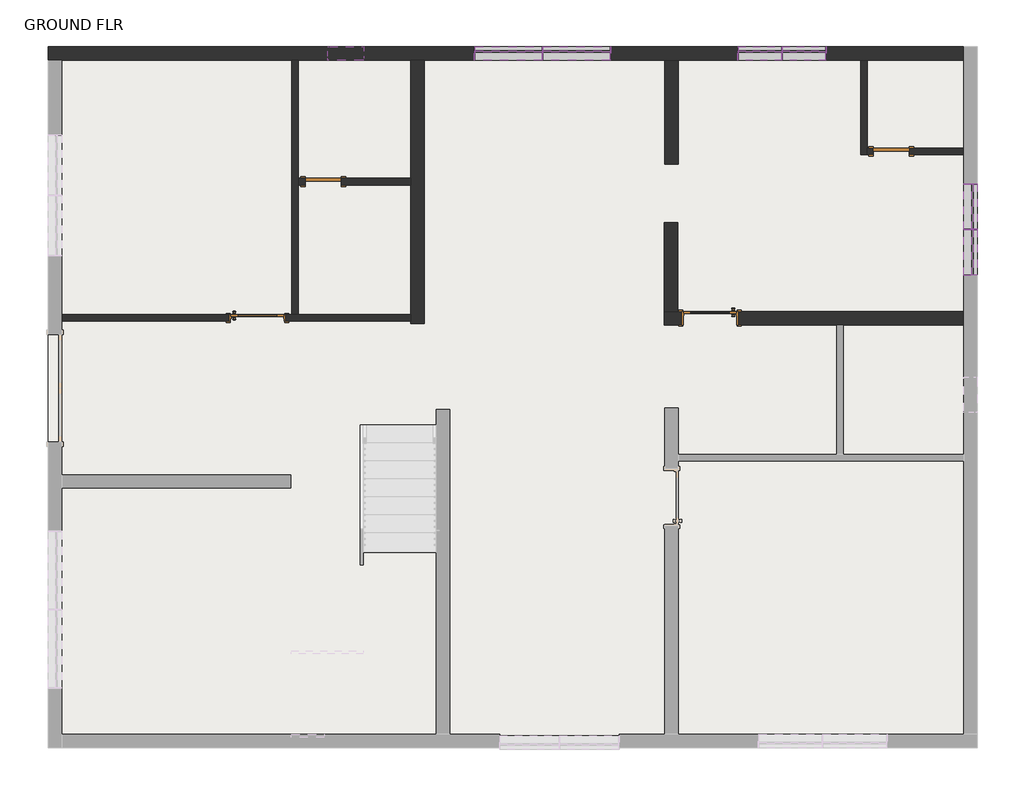
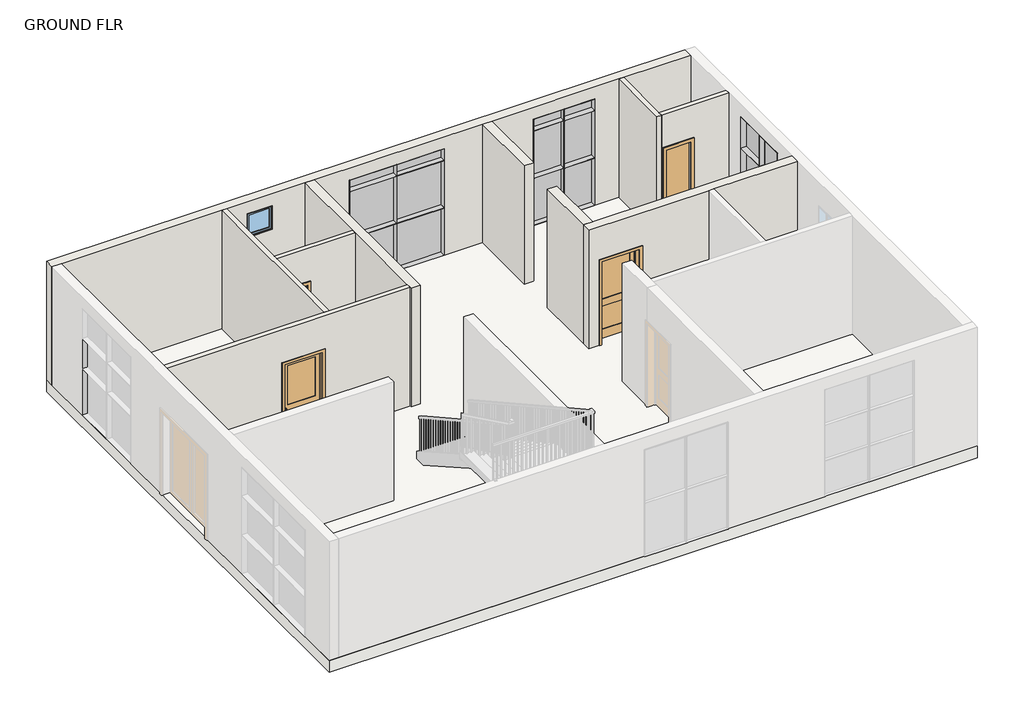
# One storey, part 2 of 3: 53 members, 18 plates, 10 walls, 4 doors, 1 slab, 1 window.
"""IFC4 building model written with IfcOpenShell, lengths in millimetres."""

from ifc_helpers import new_model, si_unit, frame, origin, origin_with_axes, place, context, project, spatial, polyline, outline, extrude, faceted_brep, transform, mapped, element, save
from components import door_interior_single_2_panel_wood_d4071c8b, door_interior_single_2_panel_wood_5dd36918, single_flush_bathroom_2_x_7_0bf9f8da, member_9b8c6d2b, member_330b65be, member_e8dc6119, member_d66a3bdd, member_a87dc375, member_05d02c6e, member_049ff311, member_f4ca0770, member_7d5ce663, member_d90fa784, member_091456ab, member_579a4f36, member_81a97153, member_446da441, member_c9ff8968, member_427a6bf5, member_b53b5e8d, member_fa9cb678, system_panel_glazed_6813505b, system_panel_glazed_75f85cfe, system_panel_glazed_a35be92d, system_panel_glazed_47c35fab, system_panel_glazed_b4a359f9, system_panel_glazed_e62deb46, system_panel_glazed_14aec0f7, system_panel_glazed_b869959d, system_panel_glazed_d22e8d08, window_80340324

model = new_model("IFC4")

# Units and contexts
model_context = context("Model", 3, world=origin())
ifc_project = project(units=[si_unit("LENGTHUNIT", "METRE", prefix="MILLI")], contexts=[model_context])

# Site, building, storey
site = spatial("IfcSite", under=ifc_project)
building = spatial("IfcBuilding", under=site)
storey = spatial("IfcBuildingStorey", under=building, Name="GROUND FLR", Elevation=304.8)

# Doors
placement = place(None, origin())
door_interior_single_2_panel_wood_shape = door_interior_single_2_panel_wood_d4071c8b(model_context)
element("IfcDoor", 1, ObjectType="Door-Interior-Single-2_Panel-Wood", at=placement, inside=storey, context=model_context, shape_type="MappedRepresentation", body=[
    mapped(door_interior_single_2_panel_wood_shape, transform((-6802.5434923, 1073.5921668, 304.8), x_axis=(1.0, 0.0, 0.0), y_axis=(0.0, 1.0, 0.0), z_axis=(0.0, 0.0, 1.0))),
])
door_interior_single_2_panel_wood_2_shape = door_interior_single_2_panel_wood_5dd36918(model_context)
element("IfcDoor", 2, ObjectType="Door-Interior-Single-2_Panel-Wood", at=placement, inside=storey, context=model_context, shape_type="MappedRepresentation", body=[
    mapped(door_interior_single_2_panel_wood_2_shape, transform((872.4132515, 1069.6301442, 304.8), x_axis=(-1.0, 0.0, 0.0), y_axis=(0.0, -1.0, 0.0), z_axis=(0.0, 0.0, 1.0))),
])
single_flush_bathroom_2_x_7_shape = single_flush_bathroom_2_x_7_0bf9f8da(model_context)
element("IfcDoor", 3, ObjectType="Single-Flush : BATHROOM 2' X 7'", at=placement, inside=storey, context=model_context, shape_type="MappedRepresentation", body=[
    mapped(single_flush_bathroom_2_x_7_shape, transform((-5684.9434923, 3381.9805563, 304.8), x_axis=(-1.0, 0.0, 0.0), y_axis=(0.0, -1.0, 0.0), z_axis=(0.0, 0.0, 1.0))),
])
element("IfcDoor", 4, ObjectType="Single-Flush : BATHROOM 2' X 7'", at=placement, inside=storey, context=model_context, shape_type="MappedRepresentation", body=[
    mapped(single_flush_bathroom_2_x_7_shape, transform((3941.8301763, 3897.1946858, 304.8), x_axis=(-1.0, 0.0, 0.0), y_axis=(0.0, -1.0, 0.0), z_axis=(0.0, 0.0, 1.0))),
])

# Members
member_shape = member_9b8c6d2b(model_context)
element("IfcMember", 5, ObjectType="Rectangular Mullion : 2.5\" x 5\" rectangular", at=placement, inside=storey, context=model_context, shape_type="MappedRepresentation", body=[
    mapped(member_shape, transform((-10239.065751, 4179.68206, 1498.6), x_axis=(0.0, 1.0, 0.0), y_axis=(-1.0, 0.0, 0.0), z_axis=(0.0, 0.0, 1.0))),
])
member_2_shape = member_330b65be(model_context)
element("IfcMember", 6, ObjectType="Rectangular Mullion : 2.5\" x 5\" rectangular", at=placement, inside=storey, context=model_context, shape_type="MappedRepresentation", body=[
    mapped(member_2_shape, transform((-10239.065751, 4179.68206, 2273.3), x_axis=(0.0, 1.0, 0.0), y_axis=(-1.0, 0.0, 0.0), z_axis=(0.0, 0.0, 1.0))),
])
member_3_shape = member_e8dc6119(model_context)
element("IfcMember", 7, ObjectType="Rectangular Mullion : 2.5\" x 5\" rectangular", at=placement, inside=storey, context=model_context, shape_type="MappedRepresentation", body=[
    mapped(member_3_shape, transform((5293.034249, 2571.0346634, 2235.2), x_axis=(0.0, -1.0, 0.0), y_axis=(-1.0, 0.0, 0.0), z_axis=(0.0, 0.0, -1.0))),
])
member_4_shape = member_d66a3bdd(model_context)
element("IfcMember", 8, ObjectType="Rectangular Mullion : 2.5\" x 5\" rectangular", at=placement, inside=storey, context=model_context, shape_type="MappedRepresentation", body=[
    mapped(member_4_shape, transform((5293.034249, 3348.9096634, 3048.0), x_axis=(0.0, 1.0, 0.0), y_axis=(-1.0, 0.0, 0.0), z_axis=(0.0, 0.0, 1.0))),
])
element("IfcMember", 9, ObjectType="Rectangular Mullion : 2.5\" x 5\" rectangular", at=placement, inside=storey, context=model_context, shape_type="MappedRepresentation", body=[
    mapped(member_4_shape, transform((5293.034249, 1793.1596634, 2235.2), x_axis=(0.0, -1.0, 0.0), y_axis=(-1.0, 0.0, 0.0), z_axis=(0.0, 0.0, -1.0))),
])
member_5_shape = member_a87dc375(model_context)
element("IfcMember", 10, ObjectType="Rectangular Mullion : 2.5\" x 5\" rectangular", at=placement, inside=storey, context=model_context, shape_type="MappedRepresentation", body=[
    mapped(member_5_shape, transform((5293.034249, 2571.0346634, 304.8), x_axis=(0.0, -1.0, 0.0), y_axis=(-1.0, 0.0, 0.0), z_axis=(0.0, 0.0, -1.0))),
])
member_6_shape = member_05d02c6e(model_context)
element("IfcMember", 11, ObjectType="Rectangular Mullion : 2.5\" x 5\" rectangular", at=placement, inside=storey, context=model_context, shape_type="MappedRepresentation", body=[
    mapped(member_6_shape, transform((5293.034249, 2571.0346634, 1168.4), x_axis=(0.0, -1.0, 0.0), y_axis=(-1.0, 0.0, 0.0), z_axis=(0.0, 0.0, -1.0))),
])
member_7_shape = member_049ff311(model_context)
element("IfcMember", 12, ObjectType="Rectangular Mullion : 2.5\" x 5\" rectangular", at=placement, inside=storey, context=model_context, shape_type="MappedRepresentation", body=[
    mapped(member_7_shape, transform((5293.034249, 1793.1596634, 304.8), x_axis=(0.0, -1.0, 0.0), y_axis=(-1.0, 0.0, 0.0), z_axis=(0.0, 0.0, -1.0))),
])
member_8_shape = member_f4ca0770(model_context)
element("IfcMember", 13, ObjectType="Rectangular Mullion : 2.5\" x 5\" rectangular", at=placement, inside=storey, context=model_context, shape_type="MappedRepresentation", body=[
    mapped(member_8_shape, transform((5293.034249, 3348.9096634, 2235.2), x_axis=(0.0, 1.0, 0.0), y_axis=(-1.0, 0.0, 0.0), z_axis=(0.0, 0.0, 1.0))),
])
element("IfcMember", 14, ObjectType="Rectangular Mullion : 2.5\" x 5\" rectangular", at=placement, inside=storey, context=model_context, shape_type="MappedRepresentation", body=[
    mapped(member_8_shape, transform((5293.034249, 1793.1596634, 1168.4), x_axis=(0.0, -1.0, 0.0), y_axis=(-1.0, 0.0, 0.0), z_axis=(0.0, 0.0, -1.0))),
])
element("IfcMember", 15, ObjectType="Rectangular Mullion : 2.5\" x 5\" rectangular", at=placement, inside=storey, context=model_context, shape_type="MappedRepresentation", body=[
    mapped(member_7_shape, transform((5293.034249, 3348.9096634, 1168.4), x_axis=(0.0, 1.0, 0.0), y_axis=(-1.0, 0.0, 0.0), z_axis=(0.0, 0.0, 1.0))),
])
member_9_shape = member_7d5ce663(model_context)
element("IfcMember", 16, ObjectType="Rectangular Mullion : 2.5\" x 5\" rectangular", at=placement, inside=storey, context=model_context, shape_type="MappedRepresentation", body=[
    mapped(member_9_shape, transform((-821.7324923, 5560.8946858, 3048.0), x_axis=(0.0, 0.0, 1.0), y_axis=(0.0, -1.0, 0.0), z_axis=(1.0, 0.0, 0.0))),
])
element("IfcMember", 17, ObjectType="Rectangular Mullion : 2.5\" x 5\" rectangular", at=placement, inside=storey, context=model_context, shape_type="MappedRepresentation", body=[
    mapped(member_9_shape, transform((-1973.8129923, 5560.8946858, 3048.0), x_axis=(0.0, 0.0, 1.0), y_axis=(0.0, -1.0, 0.0), z_axis=(1.0, 0.0, 0.0))),
])
element("IfcMember", 18, ObjectType="Rectangular Mullion : 2.5\" x 5\" rectangular", at=placement, inside=storey, context=model_context, shape_type="MappedRepresentation", body=[
    mapped(member_9_shape, transform((-3118.6544923, 5560.8946858, 304.8), x_axis=(0.0, 0.0, -1.0), y_axis=(0.0, -1.0, 0.0), z_axis=(-1.0, 0.0, 0.0))),
])
element("IfcMember", 19, ObjectType="Rectangular Mullion : 2.5\" x 5\" rectangular", at=placement, inside=storey, context=model_context, shape_type="MappedRepresentation", body=[
    mapped(member_9_shape, transform((-1966.5739923, 5560.8946858, 304.8), x_axis=(0.0, 0.0, -1.0), y_axis=(0.0, -1.0, 0.0), z_axis=(-1.0, 0.0, 0.0))),
])
member_10_shape = member_d90fa784(model_context)
element("IfcMember", 20, ObjectType="Rectangular Mullion : 2.5\" x 5\" rectangular", at=placement, inside=storey, context=model_context, shape_type="MappedRepresentation", body=[
    mapped(member_10_shape, transform((5293.034249, 1800.3986634, 3048.0), x_axis=(0.0, 0.0, 1.0), y_axis=(-1.0, 0.0, 0.0), z_axis=(0.0, -1.0, 0.0))),
])
element("IfcMember", 21, ObjectType="Rectangular Mullion : 2.5\" x 5\" rectangular", at=placement, inside=storey, context=model_context, shape_type="MappedRepresentation", body=[
    mapped(member_10_shape, transform((5293.034249, 2574.6541634, 3048.0), x_axis=(0.0, 0.0, 1.0), y_axis=(-1.0, 0.0, 0.0), z_axis=(0.0, -1.0, 0.0))),
])
element("IfcMember", 22, ObjectType="Rectangular Mullion : 2.5\" x 5\" rectangular", at=placement, inside=storey, context=model_context, shape_type="MappedRepresentation", body=[
    mapped(member_10_shape, transform((5293.034249, 3341.6706634, 304.8), x_axis=(0.0, 0.0, -1.0), y_axis=(-1.0, 0.0, 0.0), z_axis=(0.0, 1.0, 0.0))),
])
element("IfcMember", 23, ObjectType="Rectangular Mullion : 2.5\" x 5\" rectangular", at=placement, inside=storey, context=model_context, shape_type="MappedRepresentation", body=[
    mapped(member_10_shape, transform((5293.034249, 2567.4151634, 304.8), x_axis=(0.0, 0.0, -1.0), y_axis=(-1.0, 0.0, 0.0), z_axis=(0.0, 1.0, 0.0))),
])
member_11_shape = member_091456ab(model_context)
element("IfcMember", 24, ObjectType="Rectangular Mullion : 2.5\" x 5\" rectangular", at=placement, inside=storey, context=model_context, shape_type="MappedRepresentation", body=[
    mapped(member_11_shape, transform((5293.034249, 2574.6541634, 2235.2), x_axis=(0.0, 0.0, 1.0), y_axis=(-1.0, 0.0, 0.0), z_axis=(0.0, -1.0, 0.0))),
])
element("IfcMember", 25, ObjectType="Rectangular Mullion : 2.5\" x 5\" rectangular", at=placement, inside=storey, context=model_context, shape_type="MappedRepresentation", body=[
    mapped(member_11_shape, transform((5293.034249, 1800.3986634, 2235.2), x_axis=(0.0, 0.0, 1.0), y_axis=(-1.0, 0.0, 0.0), z_axis=(0.0, -1.0, 0.0))),
])
element("IfcMember", 26, ObjectType="Rectangular Mullion : 2.5\" x 5\" rectangular", at=placement, inside=storey, context=model_context, shape_type="MappedRepresentation", body=[
    mapped(member_11_shape, transform((5293.034249, 2574.6541634, 1168.4), x_axis=(0.0, 0.0, 1.0), y_axis=(-1.0, 0.0, 0.0), z_axis=(0.0, -1.0, 0.0))),
])
element("IfcMember", 27, ObjectType="Rectangular Mullion : 2.5\" x 5\" rectangular", at=placement, inside=storey, context=model_context, shape_type="MappedRepresentation", body=[
    mapped(member_11_shape, transform((5293.034249, 1800.3986634, 1168.4), x_axis=(0.0, 0.0, 1.0), y_axis=(-1.0, 0.0, 0.0), z_axis=(0.0, -1.0, 0.0))),
])
member_12_shape = member_579a4f36(model_context)
element("IfcMember", 28, ObjectType="Rectangular Mullion : 2.5\" x 5\" rectangular", at=placement, inside=storey, context=model_context, shape_type="MappedRepresentation", body=[
    mapped(member_12_shape, transform((2845.1337936, 5560.8946858, 2743.2), x_axis=(1.0, 0.0, 0.0), y_axis=(0.0, -1.0, 0.0), z_axis=(0.0, 0.0, -1.0))),
])
element("IfcMember", 29, ObjectType="Rectangular Mullion : 2.5\" x 5\" rectangular", at=placement, inside=storey, context=model_context, shape_type="MappedRepresentation", body=[
    mapped(member_12_shape, transform((-814.4934923, 5560.8946858, 2743.2), x_axis=(1.0, 0.0, 0.0), y_axis=(0.0, -1.0, 0.0), z_axis=(0.0, 0.0, -1.0))),
])
element("IfcMember", 30, ObjectType="Rectangular Mullion : 2.5\" x 5\" rectangular", at=placement, inside=storey, context=model_context, shape_type="MappedRepresentation", body=[
    mapped(member_12_shape, transform((-3125.8934923, 5560.8946858, 3048.0), x_axis=(-1.0, 0.0, 0.0), y_axis=(0.0, -1.0, 0.0), z_axis=(0.0, 0.0, 1.0))),
])
element("IfcMember", 31, ObjectType="Rectangular Mullion : 2.5\" x 5\" rectangular", at=placement, inside=storey, context=model_context, shape_type="MappedRepresentation", body=[
    mapped(member_12_shape, transform((1346.5337936, 5560.8946858, 3048.0), x_axis=(-1.0, 0.0, 0.0), y_axis=(0.0, -1.0, 0.0), z_axis=(0.0, 0.0, 1.0))),
])
member_13_shape = member_81a97153(model_context)
element("IfcMember", 32, ObjectType="Rectangular Mullion : 2.5\" x 5\" rectangular", at=placement, inside=storey, context=model_context, shape_type="MappedRepresentation", body=[
    mapped(member_13_shape, transform((-814.4934923, 5560.8946858, 304.8), x_axis=(1.0, 0.0, 0.0), y_axis=(0.0, -1.0, 0.0), z_axis=(0.0, 0.0, -1.0))),
])
element("IfcMember", 33, ObjectType="Rectangular Mullion : 2.5\" x 5\" rectangular", at=placement, inside=storey, context=model_context, shape_type="MappedRepresentation", body=[
    mapped(member_13_shape, transform((2845.1337936, 5560.8946858, 304.8), x_axis=(1.0, 0.0, 0.0), y_axis=(0.0, -1.0, 0.0), z_axis=(0.0, 0.0, -1.0))),
])
element("IfcMember", 34, ObjectType="Rectangular Mullion : 2.5\" x 5\" rectangular", at=placement, inside=storey, context=model_context, shape_type="MappedRepresentation", body=[
    mapped(member_13_shape, transform((1346.5337936, 5560.8946858, 2743.2), x_axis=(-1.0, 0.0, 0.0), y_axis=(0.0, -1.0, 0.0), z_axis=(0.0, 0.0, 1.0))),
])
element("IfcMember", 35, ObjectType="Rectangular Mullion : 2.5\" x 5\" rectangular", at=placement, inside=storey, context=model_context, shape_type="MappedRepresentation", body=[
    mapped(member_13_shape, transform((-3125.8934923, 5560.8946858, 2743.2), x_axis=(-1.0, 0.0, 0.0), y_axis=(0.0, -1.0, 0.0), z_axis=(0.0, 0.0, 1.0))),
])
element("IfcMember", 36, ObjectType="Rectangular Mullion : 2.5\" x 5\" rectangular", at=placement, inside=storey, context=model_context, shape_type="MappedRepresentation", body=[
    mapped(member_13_shape, transform((2845.1337936, 5560.8946858, 1524.0), x_axis=(1.0, 0.0, 0.0), y_axis=(0.0, -1.0, 0.0), z_axis=(0.0, 0.0, -1.0))),
])
element("IfcMember", 37, ObjectType="Rectangular Mullion : 2.5\" x 5\" rectangular", at=placement, inside=storey, context=model_context, shape_type="MappedRepresentation", body=[
    mapped(member_13_shape, transform((-814.4934923, 5560.8946858, 1524.0), x_axis=(1.0, 0.0, 0.0), y_axis=(0.0, -1.0, 0.0), z_axis=(0.0, 0.0, -1.0))),
])
element("IfcMember", 38, ObjectType="Rectangular Mullion : 2.5\" x 5\" rectangular", at=placement, inside=storey, context=model_context, shape_type="MappedRepresentation", body=[
    mapped(member_13_shape, transform((1346.5337936, 5560.8946858, 1524.0), x_axis=(-1.0, 0.0, 0.0), y_axis=(0.0, -1.0, 0.0), z_axis=(0.0, 0.0, 1.0))),
])
element("IfcMember", 39, ObjectType="Rectangular Mullion : 2.5\" x 5\" rectangular", at=placement, inside=storey, context=model_context, shape_type="MappedRepresentation", body=[
    mapped(member_13_shape, transform((-3125.8934923, 5560.8946858, 1524.0), x_axis=(-1.0, 0.0, 0.0), y_axis=(0.0, -1.0, 0.0), z_axis=(0.0, 0.0, 1.0))),
])
member_14_shape = member_446da441(model_context)
element("IfcMember", 40, ObjectType="Rectangular Mullion : 2.5\" x 5\" rectangular", at=placement, inside=storey, context=model_context, shape_type="MappedRepresentation", body=[
    mapped(member_14_shape, transform((2837.8947936, 5560.8946858, 3048.0), x_axis=(0.0, 0.0, 1.0), y_axis=(0.0, -1.0, 0.0), z_axis=(1.0, 0.0, 0.0))),
])
element("IfcMember", 41, ObjectType="Rectangular Mullion : 2.5\" x 5\" rectangular", at=placement, inside=storey, context=model_context, shape_type="MappedRepresentation", body=[
    mapped(member_14_shape, transform((2092.2142936, 5560.8946858, 3048.0), x_axis=(0.0, 0.0, 1.0), y_axis=(0.0, -1.0, 0.0), z_axis=(1.0, 0.0, 0.0))),
])
element("IfcMember", 42, ObjectType="Rectangular Mullion : 2.5\" x 5\" rectangular", at=placement, inside=storey, context=model_context, shape_type="MappedRepresentation", body=[
    mapped(member_14_shape, transform((1353.7727936, 5560.8946858, 304.8), x_axis=(0.0, 0.0, -1.0), y_axis=(0.0, -1.0, 0.0), z_axis=(-1.0, 0.0, 0.0))),
])
element("IfcMember", 43, ObjectType="Rectangular Mullion : 2.5\" x 5\" rectangular", at=placement, inside=storey, context=model_context, shape_type="MappedRepresentation", body=[
    mapped(member_14_shape, transform((2099.4532936, 5560.8946858, 304.8), x_axis=(0.0, 0.0, -1.0), y_axis=(0.0, -1.0, 0.0), z_axis=(-1.0, 0.0, 0.0))),
])
member_15_shape = member_c9ff8968(model_context)
element("IfcMember", 44, ObjectType="Rectangular Mullion : 2.5\" x 5\" rectangular", at=placement, inside=storey, context=model_context, shape_type="MappedRepresentation", body=[
    mapped(member_15_shape, transform((2092.2142936, 5560.8946858, 2743.2), x_axis=(0.0, 0.0, 1.0), y_axis=(0.0, -1.0, 0.0), z_axis=(1.0, 0.0, 0.0))),
])
element("IfcMember", 45, ObjectType="Rectangular Mullion : 2.5\" x 5\" rectangular", at=placement, inside=storey, context=model_context, shape_type="MappedRepresentation", body=[
    mapped(member_15_shape, transform((2092.2142936, 5560.8946858, 1524.0), x_axis=(0.0, 0.0, 1.0), y_axis=(0.0, -1.0, 0.0), z_axis=(1.0, 0.0, 0.0))),
])
element("IfcMember", 46, ObjectType="Rectangular Mullion : 2.5\" x 5\" rectangular", at=placement, inside=storey, context=model_context, shape_type="MappedRepresentation", body=[
    mapped(member_15_shape, transform((2837.8947936, 5560.8946858, 1524.0), x_axis=(0.0, 0.0, 1.0), y_axis=(0.0, -1.0, 0.0), z_axis=(1.0, 0.0, 0.0))),
])
element("IfcMember", 47, ObjectType="Rectangular Mullion : 2.5\" x 5\" rectangular", at=placement, inside=storey, context=model_context, shape_type="MappedRepresentation", body=[
    mapped(member_15_shape, transform((2837.8947936, 5560.8946858, 2743.2), x_axis=(0.0, 0.0, 1.0), y_axis=(0.0, -1.0, 0.0), z_axis=(1.0, 0.0, 0.0))),
])
member_16_shape = member_427a6bf5(model_context)
element("IfcMember", 48, ObjectType="Rectangular Mullion : 2.5\" x 5\" rectangular", at=placement, inside=storey, context=model_context, shape_type="MappedRepresentation", body=[
    mapped(member_16_shape, transform((-1970.1934923, 5560.8946858, 304.8), x_axis=(1.0, 0.0, 0.0), y_axis=(0.0, -1.0, 0.0), z_axis=(0.0, 0.0, -1.0))),
])
element("IfcMember", 49, ObjectType="Rectangular Mullion : 2.5\" x 5\" rectangular", at=placement, inside=storey, context=model_context, shape_type="MappedRepresentation", body=[
    mapped(member_16_shape, transform((2095.8337936, 5560.8946858, 304.8), x_axis=(1.0, 0.0, 0.0), y_axis=(0.0, -1.0, 0.0), z_axis=(0.0, 0.0, -1.0))),
])
element("IfcMember", 50, ObjectType="Rectangular Mullion : 2.5\" x 5\" rectangular", at=placement, inside=storey, context=model_context, shape_type="MappedRepresentation", body=[
    mapped(member_16_shape, transform((2095.8337936, 5560.8946858, 1524.0), x_axis=(1.0, 0.0, 0.0), y_axis=(0.0, -1.0, 0.0), z_axis=(0.0, 0.0, -1.0))),
])
element("IfcMember", 51, ObjectType="Rectangular Mullion : 2.5\" x 5\" rectangular", at=placement, inside=storey, context=model_context, shape_type="MappedRepresentation", body=[
    mapped(member_16_shape, transform((-1970.1934923, 5560.8946858, 1524.0), x_axis=(1.0, 0.0, 0.0), y_axis=(0.0, -1.0, 0.0), z_axis=(0.0, 0.0, -1.0))),
])
member_17_shape = member_b53b5e8d(model_context)
element("IfcMember", 52, ObjectType="Rectangular Mullion : 2.5\" x 5\" rectangular", at=placement, inside=storey, context=model_context, shape_type="MappedRepresentation", body=[
    mapped(member_17_shape, transform((2095.8337936, 5560.8946858, 2743.2), x_axis=(1.0, 0.0, 0.0), y_axis=(0.0, -1.0, 0.0), z_axis=(0.0, 0.0, -1.0))),
])
element("IfcMember", 53, ObjectType="Rectangular Mullion : 2.5\" x 5\" rectangular", at=placement, inside=storey, context=model_context, shape_type="MappedRepresentation", body=[
    mapped(member_17_shape, transform((-1970.1934923, 5560.8946858, 2743.2), x_axis=(1.0, 0.0, 0.0), y_axis=(0.0, -1.0, 0.0), z_axis=(0.0, 0.0, -1.0))),
])
member_18_shape = member_fa9cb678(model_context)
element("IfcMember", 54, ObjectType="Rectangular Mullion : 2.5\" x 5\" rectangular", at=placement, inside=storey, context=model_context, shape_type="MappedRepresentation", body=[
    mapped(member_18_shape, transform((-1973.8129923, 5560.8946858, 2743.2), x_axis=(0.0, 0.0, 1.0), y_axis=(0.0, -1.0, 0.0), z_axis=(1.0, 0.0, 0.0))),
])
element("IfcMember", 55, ObjectType="Rectangular Mullion : 2.5\" x 5\" rectangular", at=placement, inside=storey, context=model_context, shape_type="MappedRepresentation", body=[
    mapped(member_18_shape, transform((-821.7324923, 5560.8946858, 2743.2), x_axis=(0.0, 0.0, 1.0), y_axis=(0.0, -1.0, 0.0), z_axis=(1.0, 0.0, 0.0))),
])
element("IfcMember", 56, ObjectType="Rectangular Mullion : 2.5\" x 5\" rectangular", at=placement, inside=storey, context=model_context, shape_type="MappedRepresentation", body=[
    mapped(member_18_shape, transform((-1973.8129923, 5560.8946858, 1524.0), x_axis=(0.0, 0.0, 1.0), y_axis=(0.0, -1.0, 0.0), z_axis=(1.0, 0.0, 0.0))),
])
element("IfcMember", 57, ObjectType="Rectangular Mullion : 2.5\" x 5\" rectangular", at=placement, inside=storey, context=model_context, shape_type="MappedRepresentation", body=[
    mapped(member_18_shape, transform((-821.7324923, 5560.8946858, 1524.0), x_axis=(0.0, 0.0, 1.0), y_axis=(0.0, -1.0, 0.0), z_axis=(1.0, 0.0, 0.0))),
])

# Plates
system_panel_glazed_shape = system_panel_glazed_6813505b(model_context)
element("IfcPlate", 58, ObjectType="System Panel : Glazed", at=placement, inside=storey, context=model_context, shape_type="MappedRepresentation", body=[
    mapped(system_panel_glazed_shape, transform((5293.034249, 2958.1624134, 312.039), x_axis=(0.0, -1.0, 0.0), y_axis=(1.0, 0.0, 0.0), z_axis=(0.0, 0.0, 1.0))),
])
element("IfcPlate", 59, ObjectType="System Panel : Glazed", at=placement, inside=storey, context=model_context, shape_type="MappedRepresentation", body=[
    mapped(system_panel_glazed_shape, transform((5293.034249, 2183.9069134, 312.039), x_axis=(0.0, -1.0, 0.0), y_axis=(1.0, 0.0, 0.0), z_axis=(0.0, 0.0, 1.0))),
])
system_panel_glazed_2_shape = system_panel_glazed_75f85cfe(model_context)
element("IfcPlate", 60, ObjectType="System Panel : Glazed", at=placement, inside=storey, context=model_context, shape_type="MappedRepresentation", body=[
    mapped(system_panel_glazed_2_shape, transform((5293.034249, 2958.1624134, 2238.8195), x_axis=(0.0, -1.0, 0.0), y_axis=(1.0, 0.0, 0.0), z_axis=(0.0, 0.0, 1.0))),
])
element("IfcPlate", 61, ObjectType="System Panel : Glazed", at=placement, inside=storey, context=model_context, shape_type="MappedRepresentation", body=[
    mapped(system_panel_glazed_2_shape, transform((5293.034249, 2183.9069134, 2238.8195), x_axis=(0.0, -1.0, 0.0), y_axis=(1.0, 0.0, 0.0), z_axis=(0.0, 0.0, 1.0))),
])
system_panel_glazed_3_shape = system_panel_glazed_a35be92d(model_context)
element("IfcPlate", 62, ObjectType="System Panel : Glazed", at=placement, inside=storey, context=model_context, shape_type="MappedRepresentation", body=[
    mapped(system_panel_glazed_3_shape, transform((5293.034249, 2958.1624134, 1172.0195), x_axis=(0.0, -1.0, 0.0), y_axis=(1.0, 0.0, 0.0), z_axis=(0.0, 0.0, 1.0))),
])
element("IfcPlate", 63, ObjectType="System Panel : Glazed", at=placement, inside=storey, context=model_context, shape_type="MappedRepresentation", body=[
    mapped(system_panel_glazed_3_shape, transform((5293.034249, 2183.9069134, 1172.0195), x_axis=(0.0, -1.0, 0.0), y_axis=(1.0, 0.0, 0.0), z_axis=(0.0, 0.0, 1.0))),
])
system_panel_glazed_4_shape = system_panel_glazed_47c35fab(model_context)
element("IfcPlate", 64, ObjectType="System Panel : Glazed", at=placement, inside=storey, context=model_context, shape_type="MappedRepresentation", body=[
    mapped(system_panel_glazed_4_shape, transform((1722.9935436, 5560.8946858, 312.039), x_axis=(1.0, 0.0, 0.0), y_axis=(0.0, 1.0, 0.0), z_axis=(0.0, 0.0, 1.0))),
])
element("IfcPlate", 65, ObjectType="System Panel : Glazed", at=placement, inside=storey, context=model_context, shape_type="MappedRepresentation", body=[
    mapped(system_panel_glazed_4_shape, transform((2468.6740436, 5560.8946858, 312.039), x_axis=(1.0, 0.0, 0.0), y_axis=(0.0, 1.0, 0.0), z_axis=(0.0, 0.0, 1.0))),
])
system_panel_glazed_5_shape = system_panel_glazed_b4a359f9(model_context)
element("IfcPlate", 66, ObjectType="System Panel : Glazed", at=placement, inside=storey, context=model_context, shape_type="MappedRepresentation", body=[
    mapped(system_panel_glazed_5_shape, transform((1722.9935436, 5560.8946858, 2746.8195), x_axis=(1.0, 0.0, 0.0), y_axis=(0.0, 1.0, 0.0), z_axis=(0.0, 0.0, 1.0))),
])
element("IfcPlate", 67, ObjectType="System Panel : Glazed", at=placement, inside=storey, context=model_context, shape_type="MappedRepresentation", body=[
    mapped(system_panel_glazed_5_shape, transform((2468.6740436, 5560.8946858, 2746.8195), x_axis=(1.0, 0.0, 0.0), y_axis=(0.0, 1.0, 0.0), z_axis=(0.0, 0.0, 1.0))),
])
system_panel_glazed_6_shape = system_panel_glazed_e62deb46(model_context)
element("IfcPlate", 68, ObjectType="System Panel : Glazed", at=placement, inside=storey, context=model_context, shape_type="MappedRepresentation", body=[
    mapped(system_panel_glazed_6_shape, transform((1722.9935436, 5560.8946858, 1527.6195), x_axis=(1.0, 0.0, 0.0), y_axis=(0.0, 1.0, 0.0), z_axis=(0.0, 0.0, 1.0))),
])
element("IfcPlate", 69, ObjectType="System Panel : Glazed", at=placement, inside=storey, context=model_context, shape_type="MappedRepresentation", body=[
    mapped(system_panel_glazed_6_shape, transform((2468.6740436, 5560.8946858, 1527.6195), x_axis=(1.0, 0.0, 0.0), y_axis=(0.0, 1.0, 0.0), z_axis=(0.0, 0.0, 1.0))),
])
system_panel_glazed_7_shape = system_panel_glazed_14aec0f7(model_context)
element("IfcPlate", 70, ObjectType="System Panel : Glazed", at=placement, inside=storey, context=model_context, shape_type="MappedRepresentation", body=[
    mapped(system_panel_glazed_7_shape, transform((-2546.2337423, 5560.8946858, 2746.8195), x_axis=(1.0, 0.0, 0.0), y_axis=(0.0, 1.0, 0.0), z_axis=(0.0, 0.0, 1.0))),
])
element("IfcPlate", 71, ObjectType="System Panel : Glazed", at=placement, inside=storey, context=model_context, shape_type="MappedRepresentation", body=[
    mapped(system_panel_glazed_7_shape, transform((-1394.1532423, 5560.8946858, 2746.8195), x_axis=(1.0, 0.0, 0.0), y_axis=(0.0, 1.0, 0.0), z_axis=(0.0, 0.0, 1.0))),
])
system_panel_glazed_8_shape = system_panel_glazed_b869959d(model_context)
element("IfcPlate", 72, ObjectType="System Panel : Glazed", at=placement, inside=storey, context=model_context, shape_type="MappedRepresentation", body=[
    mapped(system_panel_glazed_8_shape, transform((-2546.2337423, 5560.8946858, 1527.6195), x_axis=(1.0, 0.0, 0.0), y_axis=(0.0, 1.0, 0.0), z_axis=(0.0, 0.0, 1.0))),
])
element("IfcPlate", 73, ObjectType="System Panel : Glazed", at=placement, inside=storey, context=model_context, shape_type="MappedRepresentation", body=[
    mapped(system_panel_glazed_8_shape, transform((-1394.1532423, 5560.8946858, 1527.6195), x_axis=(1.0, 0.0, 0.0), y_axis=(0.0, 1.0, 0.0), z_axis=(0.0, 0.0, 1.0))),
])
system_panel_glazed_9_shape = system_panel_glazed_d22e8d08(model_context)
element("IfcPlate", 74, ObjectType="System Panel : Glazed", at=placement, inside=storey, context=model_context, shape_type="MappedRepresentation", body=[
    mapped(system_panel_glazed_9_shape, transform((-2546.2337423, 5560.8946858, 312.039), x_axis=(1.0, 0.0, 0.0), y_axis=(0.0, 1.0, 0.0), z_axis=(0.0, 0.0, 1.0))),
])
element("IfcPlate", 75, ObjectType="System Panel : Glazed", at=placement, inside=storey, context=model_context, shape_type="MappedRepresentation", body=[
    mapped(system_panel_glazed_9_shape, transform((-1394.1532423, 5560.8946858, 312.039), x_axis=(1.0, 0.0, 0.0), y_axis=(0.0, 1.0, 0.0), z_axis=(0.0, 0.0, 1.0))),
])

# Slab
element("IfcSlab", 76, ObjectType="MARBLE FLOORING 1'", at=placement, inside=storey, context=model_context, shape_type="SweptSolid", body=[
    extrude(outline(polyline([(5407.334249, 5675.1946858), (5407.334249, -6224.7053142), (-10353.365751, -6224.7053142), (-10353.365751, 5675.1946858), (5407.334249, 5675.1946858)])), origin_with_axes(), (0.0, 0.0, 1.0), 304.8),
])

# Walls
element("IfcWall", 77, at=placement, inside=storey, context=model_context, shape_type="Brep", body=[
    faceted_brep([(-10353.365751, 5675.1946858, 3352.8), (5178.734249, 5675.1946858, 3352.8), (5178.734249, 5675.1946858, 304.8), (2845.1337936, 5675.1946858, 304.8), (2845.1337936, 5675.1946858, 3048.0), (1346.5337936, 5675.1946858, 3048.0), (1346.5337936, 5675.1946858, 304.8), (-814.4934923, 5675.1946858, 304.8), (-814.4934923, 5675.1946858, 3048.0), (-3125.8934923, 5675.1946858, 3048.0), (-3125.8934923, 5675.1946858, 304.8), (-10353.365751, 5675.1946858, 304.8), (-5608.7434923, 5675.1946858, 3048.0), (-5608.7434923, 5675.1946858, 2438.4), (-4999.1434923, 5675.1946858, 2438.4), (-4999.1434923, 5675.1946858, 3048.0), (5178.734249, 5446.5946858, 3352.8), (3541.7801763, 5446.5946858, 3352.8), (3427.4801763, 5446.5946858, 3352.8), (335.7520146, 5446.5946858, 3352.8), (107.1520146, 5446.5946858, 3352.8), (-3976.7934923, 5446.5946858, 3352.8), (-4205.3934923, 5446.5946858, 3352.8), (-6110.3934923, 5446.5946858, 3352.8), (-6224.6934923, 5446.5946858, 3352.8), (-10124.765751, 5446.5946858, 3352.8), (-10353.365751, 5446.5946858, 3352.8), (-10353.365751, 5446.5946858, 304.8), (-10124.765751, 5446.5946858, 304.8), (-6224.6934923, 5446.5946858, 304.8), (-6110.3934923, 5446.5946858, 304.8), (-4205.3934923, 5446.5946858, 304.8), (-3976.7934923, 5446.5946858, 304.8), (-3125.8934923, 5446.5946858, 304.8), (-3125.8934923, 5446.5946858, 3048.0), (-814.4934923, 5446.5946858, 3048.0), (-814.4934923, 5446.5946858, 304.8), (107.1520146, 5446.5946858, 304.8), (335.7520146, 5446.5946858, 304.8), (1346.5337936, 5446.5946858, 304.8), (1346.5337936, 5446.5946858, 3048.0), (2845.1337936, 5446.5946858, 3048.0), (2845.1337936, 5446.5946858, 304.8), (3427.4801763, 5446.5946858, 304.8), (3541.7801763, 5446.5946858, 304.8), (5178.734249, 5446.5946858, 304.8), (-5608.7434923, 5446.5946858, 3048.0), (-4999.1434923, 5446.5946858, 3048.0), (-4999.1434923, 5446.5946858, 2438.4), (-5608.7434923, 5446.5946858, 2438.4)], [[[0, 1, 2, 3, 4, 5, 6, 7, 8, 9, 10, 11], [12, 13, 14, 15]], [[16, 17, 18, 19, 20, 21, 22, 23, 24, 25, 26, 27, 28, 29, 30, 31, 32, 33, 34, 35, 36, 37, 38, 39, 40, 41, 42, 43, 44, 45], [46, 47, 48, 49]], [[2, 45, 44, 43, 42, 3]], [[27, 11, 10, 33, 32, 31, 30, 29, 28]], [[36, 7, 6, 39, 38, 37]], [[1, 0, 26, 25, 24, 23, 22, 21, 20, 19, 18, 17, 16]], [[2, 1, 16, 45]], [[0, 11, 27, 26]], [[9, 34, 33, 10]], [[34, 9, 8, 35]], [[35, 8, 7, 36]], [[5, 40, 39, 6]], [[40, 5, 4, 41]], [[41, 4, 3, 42]], [[13, 12, 46, 49]], [[14, 13, 49, 48]], [[15, 14, 48, 47]], [[12, 15, 47, 46]]]),
])
element("IfcWall", 78, at=placement, inside=storey, context=model_context, shape_type="Brep", body=[
    faceted_brep([(-4205.3934923, 5446.5946858, 304.8), (-4205.3934923, 3439.1305563, 304.8), (-4205.3934923, 3324.8305563, 304.8), (-4205.3934923, 1127.5671668, 304.8), (-4205.3934923, 1013.2671668, 304.8), (-4205.3934923, 976.1946858, 304.8), (-4205.3934923, 976.1946858, 3352.8), (-4205.3934923, 1013.2671668, 3352.8), (-4205.3934923, 1127.5671668, 3352.8), (-4205.3934923, 3324.8305563, 3352.8), (-4205.3934923, 3439.1305563, 3352.8), (-4205.3934923, 5446.5946858, 3352.8), (-3976.7934923, 5446.5946858, 304.8), (-3976.7934923, 5446.5946858, 3352.8), (-3976.7934923, 976.1946858, 3352.8), (-3976.7934923, 976.1946858, 304.8)], [[[0, 1, 2, 3, 4, 5, 6, 7, 8, 9, 10, 11]], [[12, 13, 14, 15]], [[5, 4, 3, 2, 1, 0, 12, 15]], [[6, 5, 15, 14]], [[11, 10, 9, 8, 7, 6, 14, 13]], [[0, 11, 13, 12]]]),
])
element("IfcWall", 79, at=placement, inside=storey, context=model_context, shape_type="Brep", body=[
    faceted_brep([(97.7132515, 1180.7551442, 3352.8), (326.3132515, 1180.7551442, 3352.8), (5178.734249, 1180.7551442, 3352.8), (5178.734249, 1180.7551442, 304.8), (1355.0132515, 1180.7551442, 304.8), (1355.0132515, 1180.7551442, 2463.8), (389.8132515, 1180.7551442, 2463.8), (389.8132515, 1180.7551442, 304.8), (326.3132515, 1180.7551442, 304.8), (97.7132515, 1180.7551442, 304.8), (5178.734249, 952.1551442, 3352.8), (3134.034249, 952.1551442, 3352.8), (3019.734249, 952.1551442, 3352.8), (97.7132515, 952.1551442, 3352.8), (97.7132515, 952.1551442, 304.8), (389.8132515, 952.1551442, 304.8), (389.8132515, 952.1551442, 2463.8), (1355.0132515, 952.1551442, 2463.8), (1355.0132515, 952.1551442, 304.8), (3019.734249, 952.1551442, 304.8), (3134.034249, 952.1551442, 304.8), (5178.734249, 952.1551442, 304.8)], [[[0, 1, 2, 3, 4, 5, 6, 7, 8, 9]], [[10, 11, 12, 13, 14, 15, 16, 17, 18, 19, 20, 21]], [[3, 21, 20, 19, 18, 4]], [[14, 9, 8, 7, 15]], [[2, 1, 0, 13, 12, 11, 10]], [[3, 2, 10, 21]], [[0, 9, 14, 13]], [[6, 16, 15, 7]], [[16, 6, 5, 17]], [[17, 5, 4, 18]]]),
])
element("IfcWall", 80, at=placement, inside=storey, context=model_context, shape_type="SweptSolid", body=[
    extrude(outline(polyline([(107.1520146, 3681.2946858), (107.1520146, 5446.5946858), (335.7520146, 5446.5946858), (335.7520146, 3681.2946858), (107.1520146, 3681.2946858)])), frame((0.0, 0.0, 304.8), z_axis=(0.0, 0.0, 1.0), x_axis=(1.0, 0.0, 0.0)), (0.0, 0.0, 1.0), 3048.0),
])
element("IfcWall", 81, at=placement, inside=storey, context=model_context, shape_type="SweptSolid", body=[
    extrude(outline(polyline([(97.7132515, 1180.7551442), (97.7132515, 2683.528796), (326.3132515, 2683.528796), (326.3132515, 1180.7551442), (97.7132515, 1180.7551442)])), frame((0.0, 0.0, 304.8), z_axis=(0.0, 0.0, 1.0), x_axis=(1.0, 0.0, 0.0)), (0.0, 0.0, 1.0), 3048.0),
])
element("IfcWall", 82, ObjectType="INTERIOR WALL THICKNESS 4.5\"", at=placement, inside=storey, context=model_context, shape_type="Brep", body=[
    faceted_brep([(-4205.3934923, 1013.2671668, 3352.8), (-10124.765751, 1013.2671668, 3352.8), (-10124.765751, 1013.2671668, 304.8), (-7285.1434923, 1013.2671668, 304.8), (-7285.1434923, 1013.2671668, 2463.8), (-6319.9434923, 1013.2671668, 2463.8), (-6319.9434923, 1013.2671668, 304.8), (-4205.3934923, 1013.2671668, 304.8), (-10124.765751, 1127.5671668, 3352.8), (-6224.6934923, 1127.5671668, 3352.8), (-6110.3934923, 1127.5671668, 3352.8), (-4205.3934923, 1127.5671668, 3352.8), (-4205.3934923, 1127.5671668, 304.8), (-6110.3934923, 1127.5671668, 304.8), (-6224.6934923, 1127.5671668, 304.8), (-6319.9434923, 1127.5671668, 304.8), (-6319.9434923, 1127.5671668, 2463.8), (-7285.1434923, 1127.5671668, 2463.8), (-7285.1434923, 1127.5671668, 304.8), (-10124.765751, 1127.5671668, 304.8)], [[[0, 1, 2, 3, 4, 5, 6, 7]], [[8, 9, 10, 11, 12, 13, 14, 15, 16, 17, 18, 19]], [[2, 19, 18, 3]], [[12, 7, 6, 15, 14, 13]], [[1, 0, 11, 10, 9, 8]], [[2, 1, 8, 19]], [[0, 7, 12, 11]], [[5, 16, 15, 6]], [[16, 5, 4, 17]], [[17, 4, 3, 18]]]),
])
element("IfcWall", 83, ObjectType="INTERIOR WALL THICKNESS 4.5\"", at=placement, inside=storey, context=model_context, shape_type="Brep", body=[
    faceted_brep([(-6224.6934923, 5446.5946858, 304.8), (-6224.6934923, 1127.5671668, 304.8), (-6224.6934923, 1127.5671668, 3352.8), (-6224.6934923, 5446.5946858, 3352.8), (-6110.3934923, 5446.5946858, 304.8), (-6110.3934923, 5446.5946858, 3352.8), (-6110.3934923, 3439.1305563, 3352.8), (-6110.3934923, 3324.8305563, 3352.8), (-6110.3934923, 1127.5671668, 3352.8), (-6110.3934923, 1127.5671668, 304.8), (-6110.3934923, 3324.8305563, 304.8), (-6110.3934923, 3439.1305563, 304.8)], [[[0, 1, 2, 3]], [[4, 5, 6, 7, 8, 9, 10, 11]], [[1, 0, 4, 11, 10, 9]], [[3, 2, 8, 7, 6, 5]], [[0, 3, 5, 4]], [[2, 1, 9, 8]]]),
])
element("IfcWall", 84, ObjectType="INTERIOR WALL THICKNESS 4.5\"", at=placement, inside=storey, context=model_context, shape_type="SweptSolid", body=[
    extrude(outline(polyline([(304.8, -6110.3934923), (304.8, -5989.7434923), (2438.4, -5989.7434923), (2438.4, -5380.1434923), (304.8, -5380.1434923), (304.8, -4205.3934923), (3352.8, -4205.3934923), (3352.8, -6110.3934923), (304.8, -6110.3934923)])), frame((0.0, 3324.8305563, 0.0), z_axis=(0.0, 1.0, 0.0), x_axis=(0.0, 0.0, 1.0)), (0.0, 0.0, 1.0), 114.3),
])
element("IfcWall", 85, ObjectType="INTERIOR WALL THICKNESS 4.5\"", at=placement, inside=storey, context=model_context, shape_type="Brep", body=[
    faceted_brep([(3427.4801763, 5446.5946858, 304.8), (3427.4801763, 3840.0446858, 304.8), (3427.4801763, 3840.0446858, 3352.8), (3427.4801763, 5446.5946858, 3352.8), (3541.7801763, 5446.5946858, 304.8), (3541.7801763, 5446.5946858, 3352.8), (3541.7801763, 3954.3446858, 3352.8), (3541.7801763, 3840.0446858, 3352.8), (3541.7801763, 3840.0446858, 304.8), (3541.7801763, 3954.3446858, 304.8)], [[[0, 1, 2, 3]], [[4, 5, 6, 7, 8, 9]], [[1, 0, 4, 9, 8]], [[3, 2, 7, 6, 5]], [[0, 3, 5, 4]], [[2, 1, 8, 7]]]),
])
element("IfcWall", 86, ObjectType="INTERIOR WALL THICKNESS 4.5\"", at=placement, inside=storey, context=model_context, shape_type="SweptSolid", body=[
    extrude(outline(polyline([(304.8, 3541.7801763), (304.8, 3637.0301763), (2438.4, 3637.0301763), (2438.4, 4246.6301763), (304.8, 4246.6301763), (304.8, 5178.734249), (3352.8, 5178.734249), (3352.8, 3541.7801763), (304.8, 3541.7801763)])), frame((0.0, 3840.0446858, 0.0), z_axis=(0.0, 1.0, 0.0), x_axis=(0.0, 0.0, 1.0)), (0.0, 0.0, 1.0), 114.3),
])

# Window
window_shape = window_80340324(model_context)
element("IfcWindow", 87, ObjectType="Fixed : 24\" x 24\"", at=placement, inside=storey, context=model_context, shape_type="MappedRepresentation", body=[
    mapped(window_shape, transform((-5342.0434923, 5560.8946858, 1524.0), x_axis=(-1.0, 0.0, 0.0), y_axis=(0.0, -1.0, 0.0), z_axis=(0.0, 0.0, 1.0))),
])

save(model, "model.ifc")

# Revit data of these elements
# Type "Door-Interior-Single-2_Panel-Wood"
#   Type Mark = "10"
#   Assembly Code = "C1020300"
#   Analytic Construction = "Wooden"
#   Top Rail = 0' - 4 11/16"
#   Thickness = 0' - 1 3/8"
#   Thermal Resistance (R) = 2.5876 (h·ft²·°F)/BTU
#   Swing Angle [instance default] = 90.00°
#   Stiles = 0' - 4 3/4"
#   Rough Width = 3' - 2"
#   Rough Height = 7' - 1"
#   Lock Rail = 0' - 7 1/2"
#   Height = 7' - 0"
#   Width = 3' - 0"
#   Heat Transfer Coefficient (U) = 0.3865 BTU/(h·ft²·°F)
#   Bottom Rail = 0' - 9 1/8"
#   Trim Material = Cherry
#   Panel Material = Cherry
#   Frame Material = Cherry
#   Door Handle Material = Aluminum
#   Visual Light Transmittance = 0
#   Solar Heat Gain Coefficient = 0
#   Wall Closure = (empty or 0)
#   Function = (empty or 0)
# Type "Single-Flush : BATHROOM 2' X 7'"
#   Type Mark = "8"
#   Construction Type Id = "MDOOR"
#   Assembly Code = "C1020"
#   Analytic Construction = "Metal"
#   Thickness = 0' - 2"
#   Heat Transfer Coefficient (U) = 0.651978 BTU/(h·ft²·°F)
#   Height = 7' - 0"
#   Trim Projection Ext = 0' - 1"
#   Trim Projection Int = 0' - 1"
#   Trim Width = 0' - 3"
#   Width = 2' - 0"
#   Define Thermal Properties by = 1
#   Door Material = Door - Panel
#   Frame Material = Door - Frame
#   Visual Light Transmittance = 0
#   Solar Heat Gain Coefficient = 0
#   Function = (empty or 0)
#   Wall Closure = (empty or 0)
# Type "Rectangular Mullion : 2.5\" x 5\" rectangular"
#   built-in parameter 1007304 = 0.75 (stored number, unit not read)
#   built-in parameter 1007301 = 0.011875 (stored number, unit not read)
#   built-in parameter 1007300 = 0.011875 (stored number, unit not read)
# Type "System Panel : Glazed"
#   Construction Type Id = "GSP4R"
#   Analytic Construction = "1/8 in Pilkington single glazing"
#   Visual Light Transmittance = 0.9
#   Solar Heat Gain Coefficient = 0.86
#   Heat Transfer Coefficient (U) = 1.18115 BTU/(h·ft²·°F)
#   Define Thermal Properties by = 1
# Type "MARBLE FLOORING 1'"
#   Assembly Code = "B1010"
#   Function = 0
#   Layers, outside or top first: 1' - 0" "MARBLE FLOORING 1'" (function 1)
# Type
#   Assembly Code = "B2010"
#   Layers, outside or top first: 0' - 9" "BEIGE COLOUR" (function 1)
# Type "INTERIOR WALL THICKNESS 4.5\""
#   Assembly Code = "B2010"
#   Layers, outside or top first: 0' - 4 1/2" "BEIGE COLOUR" (function 1)
# Type "Fixed : 24\" x 24\""
#   Type Mark = "3"
#   Construction Type Id = "GSP4R"
#   Assembly Code = "B2020100"
#   Analytic Construction = "1/8 in Pilkington single glazing"
#   Visual Light Transmittance = 0.9
#   Solar Heat Gain Coefficient = 0.78
#   Heat Transfer Coefficient (U) = 0.6496 BTU/(h·ft²·°F)
#   Height = 2' - 0"
#   Default Sill Height = 3' - 0"
#   Width = 2' - 0"
#   Window Inset = 0' - 0 3/4"
#   Define Thermal Properties by = 1
#   Define Thermal Properties by = 1
#   Glass Pane Material = Glass
#   Sash Material = Sash
#   Wall Closure = (empty or 0)
# Elements 1, 2 (IfcDoor, "Door-Interior-Single-2_Panel-Wood")
#   Swing Angle = 90.00°
#   Phase Created = New Construction
#   Materials on its faces: "Cherry", "Aluminum"
# Elements 3, 4 (IfcDoor, "Single-Flush : BATHROOM 2' X 7'")
#   Phase Created = New Construction
#   Materials on its faces: "Door - Frame", "Door - Panel"
# Elements 5, 6, 7, 8, 9, 10, 11, 12, 13, 14, 15, 16, 17, 18, 19, 20, 21, 22, 23, 24, 25, 26, 27, 28, 29, 30, 31, 32, 33, 34, 35, 36, 37, 38, 39, 40, 41, 42, 43, 44, 45, 46, 47, 48, 49, 50, 51, 52, 53, 54, 55, 56, 57 (IfcMember, "Rectangular Mullion : 2.5\" x 5\" rectangular")
#   Phase Created = New Construction
#   Materials on its faces: "WINDOW GLASS MATERIAL"
# Elements 58, 59, 60, 61, 62, 63, 64, 65, 66, 67, 68, 69, 70, 71, 72, 73, 74, 75 (IfcPlate, "System Panel : Glazed")
#   Phase Created = New Construction
#   Materials on its faces: "Glass"
# Element 76 (IfcSlab, "MARBLE FLOORING 1'")
#   Height Offset From Level = 0' - 0"
#   Phase Created = New Construction
#   Materials on its faces: "MARBLE FLOORING 1'"
# Elements 77, 78, 79, 80, 81 (IfcWall)
#   Top Offset = 0' - 0"
#   Base Offset = 0' - 0"
#   wall height = 10' - 0"
#   Phase Created = New Construction
#   Base Constraint = GROUND FLR
#   Top Constraint = FIRST FLR
#   Materials on its faces: "BEIGE COLOUR"
# Elements 82, 83, 84, 85, 86 (IfcWall, "INTERIOR WALL THICKNESS 4.5\"")
#   Top Offset = 0' - 0"
#   Base Offset = 0' - 0"
#   wall height = 10' - 0"
#   Phase Created = New Construction
#   Base Constraint = GROUND FLR
#   Top Constraint = FIRST FLR
#   Materials on its faces: "BEIGE COLOUR"
# Element 87 (IfcWindow, "Fixed : 24\" x 24\"")
#   Mark = "1"
#   Phase Created = New Construction
#   Materials on its faces: "Sash", "Glass"
# Materials
#   "Cherry": class "Wood", colour RGB 226 177 128, transparency 0, Description = "Prunus Serotina", Cost = 0
#   "Aluminum": class "Metal", colour RGB 247 247 247, transparency 0, Description = "Aluminum 6061", Cost = 0
#   "Door - Panel": class "Wood", colour RGB 210 159 95, transparency 0, Cost = 0
#   "Door - Frame": colour RGB 118 70 51, transparency 0, Cost = 0
#   "MARBLE FLOORING 1'": class "Generic", colour RGB 120 120 120, transparency 0, Cost = 0
#   "BEIGE COLOUR": class "Generic", colour RGB 120 120 120, transparency 0, Cost = 0
#   "Glass": class "Glass", colour RGB 0 128 192, transparency 0.75, Description = "Soda Lime Glass", Cost = 0
#   "Sash": class "Wood", colour RGB 224 178 126, transparency 0, Cost = 0
#   "WINDOW GLASS MATERIAL": class "Generic", colour RGB 120 120 120, transparency 0, Cost = 0
